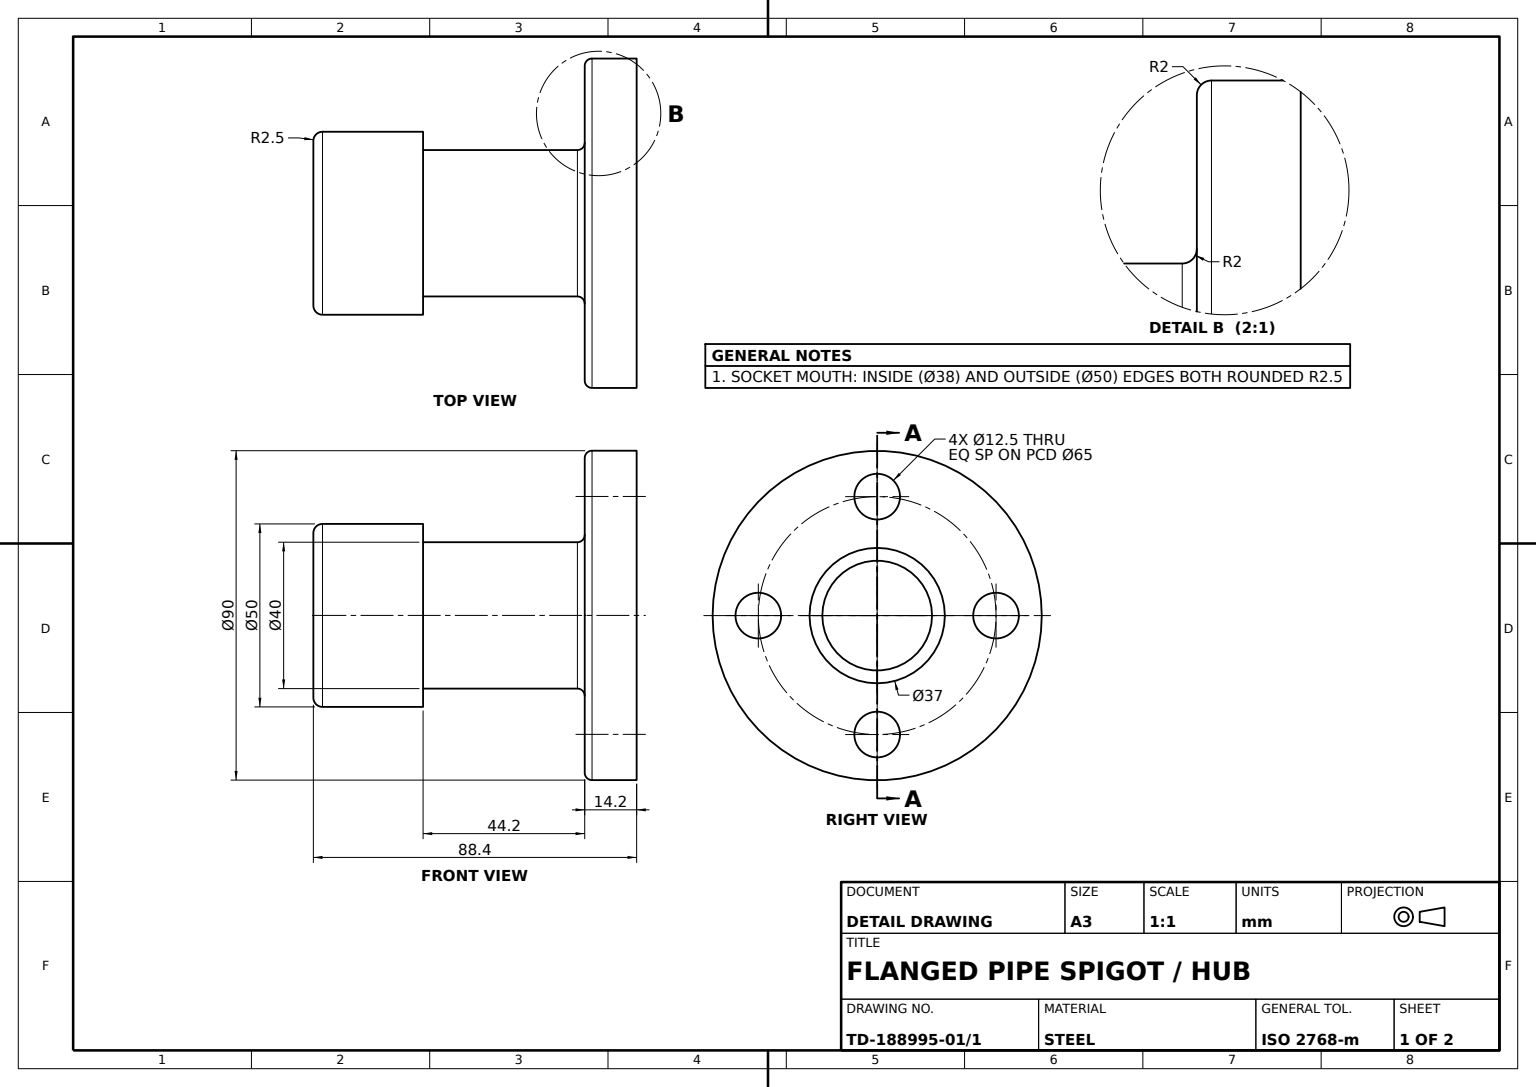
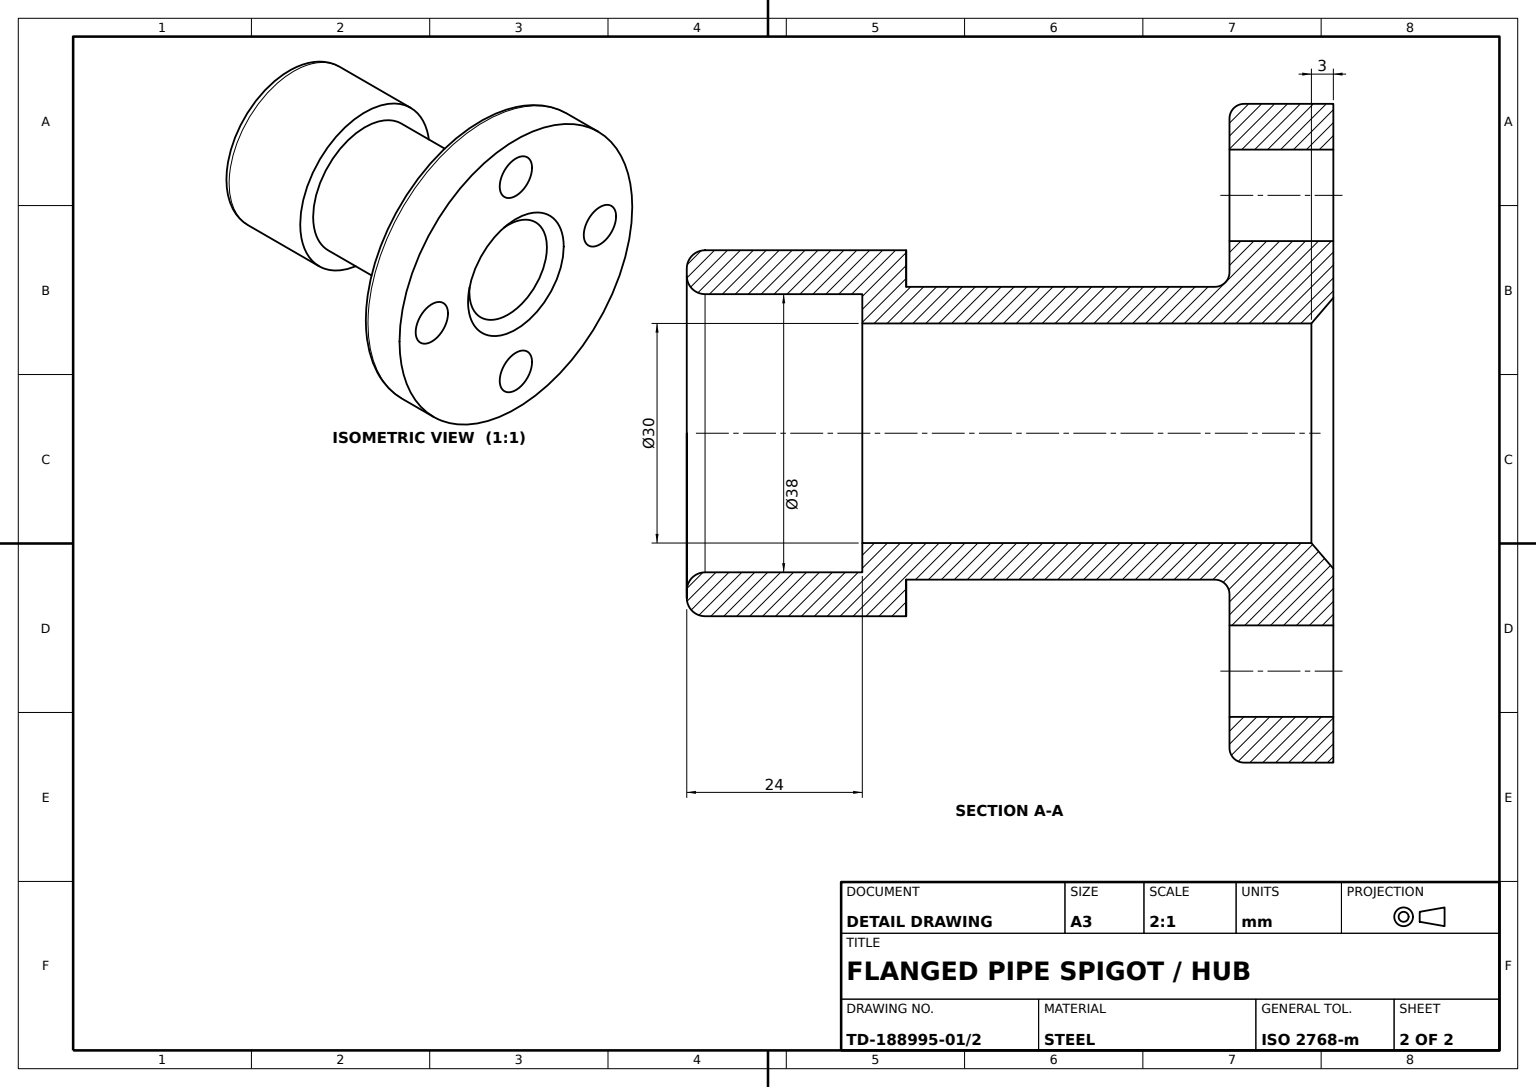
SolidWorks part; units mm, degrees
material "Plain Carbon Steel"
ref_plane "Front Plane" through (0, 0, 0) normal (0, 0, 1) x (1, 0, 0)
ref_plane "Top Plane" through (0, 0, 0) normal (0, 1, 0) x (1, 0, 0)
ref_plane "Right Plane" through (0, 0, 0) normal (1, 0, 0) x (0, 0, -1)
sketch "Flange Profile Ø90xØ30" plane through (0, 0, 0) normal (0, 0, 1) x (1, 0, 0)
  circle A0 centre (0, 0) radius 45
  circle A1 centre (0, 0) radius 15
  dimension "D1" = 90
  dimension "D2" = 30
extrude "Flange Ø90" add sketch "Flange Profile Ø90xØ30" along normal blind 14.2
sketch "Mounting Holes Sketch" plane through (0, 0, 14.2) normal (0, 0, 1) x (1, 0, 0)
  line L0 (0, 0) -> (-12.4509, 0) construction
  line L1 (0, 0) -> (0, -13.2542) construction
  circle A0 centre (0, 32.5) radius 6.25
  circle A1 centre (-32.5, 0) radius 6.25
  circle A2 centre (32.5, 0) radius 6.25
  circle A3 centre (0, -32.5) radius 6.25
  dimension "D1" = 12.5
  dimension "D2" = 12.5
  dimension "D3" = 32.5
  dimension "D4" = 32.5
extrude "Flange Mounting Holes" cut sketch "Mounting Holes Sketch" against normal through all
fillet "Flange Edge Fillet R2" radius 2 1 edges at (45, 0, 14.2)
sketch "Hub Profile Ø40xØ30" plane through (0, 0, 14.2) normal (0, 0, 1) x (1, 0, 0)
  circle A0 centre (0, 0) radius 20
  circle A1 centre (0, 0) radius 15
  dimension "D1" = 40
  dimension "D2" = 30
extrude "Hub Ø40" add sketch "Hub Profile Ø40xØ30" along normal blind 44.2
sketch "Collar Profile Ø50xØ30" plane through (0, 0, 58.4) normal (0, 0, 1) x (1, 0, 0)
  circle A0 centre (0, 0) radius 15
  circle A1 centre (0, 0) radius 25
  dimension "D1" = 30
  dimension "D2" = 50
extrude "Collar Ø50" add sketch "Collar Profile Ø50xØ30" along normal blind 6
sketch "Socket Profile Ø50xØ38" plane through (0, 0, 64.4) normal (0, 0, 1) x (1, 0, 0)
  circle A0 centre (0, 0) radius 25
  circle A1 centre (0, 0) radius 19
  dimension "D1" = 38
  dimension "D2" = 50
extrude "Socket Ø50" add sketch "Socket Profile Ø50xØ38" along normal blind 24
chamfer "Flange Chamfer" distance 3 distance2 3.5 1 edges at (15, 0, 0)
fillet "Hub Root Fillet R2" radius 2 1 edges at (20, 0, 14.2)
fillet "Socket Edge Fillet R2.5" radius 2.5 2 edges at (25, 0, 88.4) (19, 0, 88.4)
